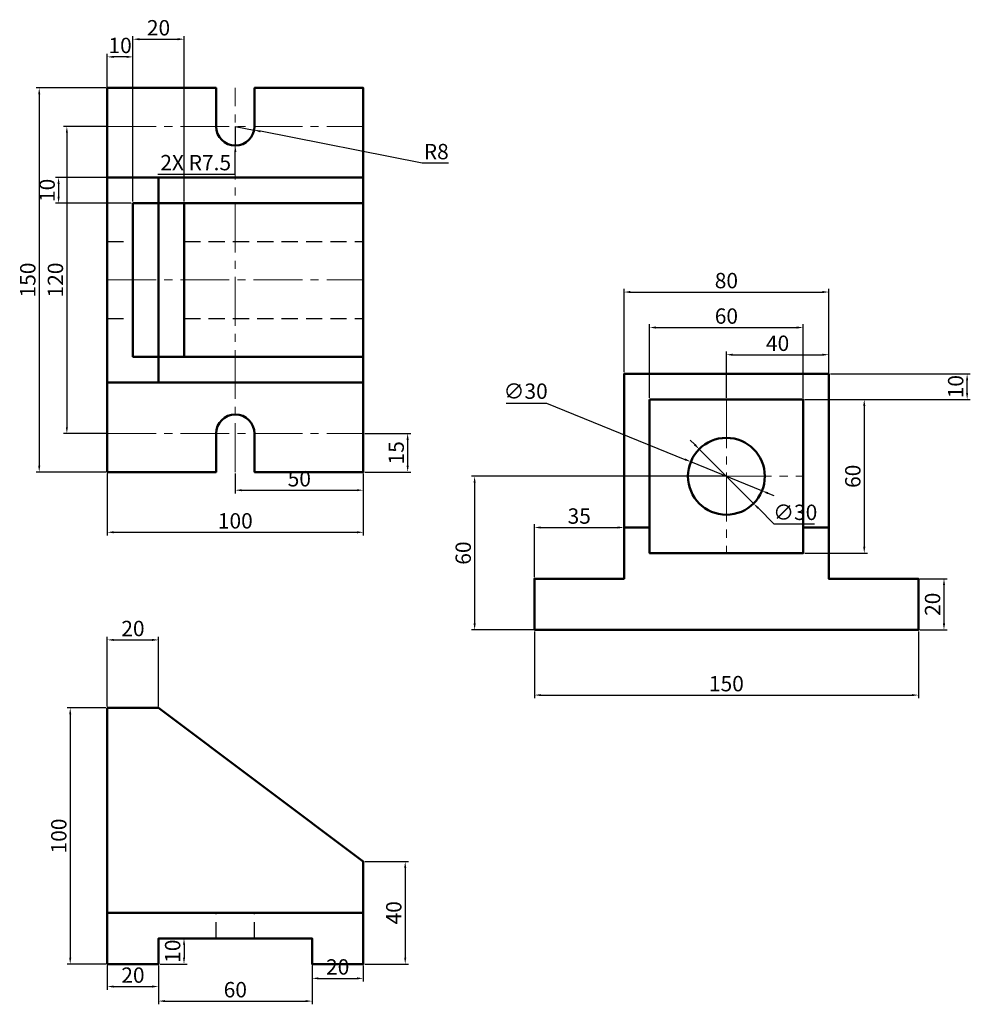
# Model space of a CAD drawing. Units: millimetres. Extents: x 18 to 390, y 656 to 1040.
import ezdxf

# ---------------------------------------------------------------- set-up
doc = ezdxf.new("R2010")
doc.units = ezdxf.units.MM
doc.linetypes.add('CENTER2', pattern=[28.575, 19.05, -3.175, 3.175, -3.175])
doc.linetypes.add('HIDDEN', pattern=[9.525, 6.35, -3.175])
for name, color, linetype, lineweight in [('M-CNTR', 4, 'CENTER2', 18), ('M-DIMS', 2, 'Continuous', 25), ('M-HIDN', 3, 'HIDDEN', 25), ('M-OUTL', 7, 'Continuous', 50)]:
    doc.layers.add(name, color=color, linetype=linetype, lineweight=lineweight)
doc.styles.get("Standard").update_dxf_attribs({"font": 'arial.ttf'})
doc.dimstyles.new('ISO-25', dxfattribs={"dimtxt": 6, "dimasz": 2.5, "dimexe": 1.25, "dimexo": 0.625, "dimtad": 1, "dimtoh": 1, "dimdec": 0, "dimtxsty": 'Standard', "dimcen": 2.5, "dimadec": 0, "dimazin": 0, "dimtfac": 1, "dimtdec": 0, "dimtmove": 0, "dimatfit": 3, "dimfxl": 1, "dimarcsym": 0})

# ---------------------------------------------------------------- blocks, each defined once
blk = doc.blocks.new('*D1')
at = {"layer": 'Defpoints', "color": 0, "transparency": 16777216}
for p in [(102.74, 998.62), (110.1, 997.18)]:
    blk.add_point(p, dxfattribs=at)
at = {"layer": 'M-DIMS', "color": 0, "lineweight": -2, "transparency": 16777216}
for p, q in [((102.74, 998.62), (110.1, 997.18)), ((175.78, 984.31), (112.55, 996.7)), ((186.09, 984.31), (175.78, 984.31))]:
    blk.add_line(p, q, dxfattribs=at)
at = {"layer": 'M-DIMS', "color": 0, "transparency": 16777216}
blk.add_solid([(112.63, 997.11), (112.47, 996.29), (110.1, 997.18)], dxfattribs=at)
at = {"layer": 'M-DIMS', "color": 0, "transparency": 16777216, "insert": (181.25, 988), "char_height": 6, "attachment_point": 5}
blk.add_mtext('R8', dxfattribs=at)
blk = doc.blocks.new('*D2')
at = {"layer": 'Defpoints', "color": 0, "transparency": 16777216}
for p in [(52.74, 1025.77), (52.74, 968.62), (62.74, 968.62)]:
    blk.add_point(p, dxfattribs=at)
at = {"layer": 'M-DIMS', "color": 0, "lineweight": -2, "transparency": 16777216}
for p, q in [((52.74, 969.24), (52.74, 1027.02)), ((62.74, 969.24), (62.74, 1027.02)), ((60.24, 1025.77), (55.24, 1025.77))]:
    blk.add_line(p, q, dxfattribs=at)
at = {"layer": 'M-DIMS', "color": 0, "transparency": 16777216}
for points in [[(55.24, 1026.19), (55.24, 1025.35), (52.74, 1025.77)], [(60.24, 1026.19), (60.24, 1025.35), (62.74, 1025.77)]]:
    blk.add_solid(points, dxfattribs=at)
at = {"layer": 'M-DIMS', "color": 0, "transparency": 16777216, "insert": (57.74, 1029.46), "char_height": 6, "attachment_point": 5}
blk.add_mtext('10', dxfattribs=at)
blk = doc.blocks.new('*D3')
at = {"layer": 'Defpoints', "color": 0, "transparency": 16777216}
for p in [(52.74, 1013.62), (26.13, 863.62), (52.74, 863.62)]:
    blk.add_point(p, dxfattribs=at)
at = {"layer": 'M-DIMS', "color": 0, "lineweight": -2, "transparency": 16777216}
for p, q in [((52.11, 1013.62), (24.88, 1013.62)), ((26.13, 1011.12), (26.13, 866.12)), ((52.11, 863.62), (24.88, 863.62))]:
    blk.add_line(p, q, dxfattribs=at)
at = {"layer": 'M-DIMS', "color": 0, "transparency": 16777216}
for points in [[(25.71, 1011.12), (26.54, 1011.12), (26.13, 1013.62)], [(25.71, 866.12), (26.54, 866.12), (26.13, 863.62)]]:
    blk.add_solid(points, dxfattribs=at)
at = {"layer": 'M-DIMS', "color": 0, "transparency": 16777216, "insert": (22.44, 938.62), "char_height": 6, "attachment_point": 5, "rotation": 90}
blk.add_mtext('150', dxfattribs=at)
blk = doc.blocks.new('*D4')
at = {"layer": 'Defpoints', "color": 0, "transparency": 16777216}
for p in [(52.74, 998.62), (36.93, 878.62), (52.74, 878.62)]:
    blk.add_point(p, dxfattribs=at)
at = {"layer": 'M-DIMS', "color": 0, "lineweight": -2, "transparency": 16777216}
for p, q in [((52.11, 998.62), (35.68, 998.62)), ((36.93, 996.12), (36.93, 881.12)), ((52.11, 878.62), (35.68, 878.62))]:
    blk.add_line(p, q, dxfattribs=at)
at = {"layer": 'M-DIMS', "color": 0, "transparency": 16777216}
for points in [[(36.52, 996.12), (37.35, 996.12), (36.93, 998.62)], [(36.52, 881.12), (37.35, 881.12), (36.93, 878.62)]]:
    blk.add_solid(points, dxfattribs=at)
at = {"layer": 'M-DIMS', "color": 0, "transparency": 16777216, "insert": (33.24, 938.62), "char_height": 6, "attachment_point": 5, "rotation": 90}
blk.add_mtext('120', dxfattribs=at)
blk = doc.blocks.new('*D5')
at = {"layer": 'Defpoints', "color": 0, "transparency": 16777216}
for p in [(102.74, 863.62), (152.74, 863.62), (152.74, 856.52)]:
    blk.add_point(p, dxfattribs=at)
at = {"layer": 'M-DIMS', "color": 0, "lineweight": -2, "transparency": 16777216}
for p, q in [((102.74, 862.99), (102.74, 855.27)), ((152.74, 862.99), (152.74, 855.27)), ((105.24, 856.52), (150.24, 856.52))]:
    blk.add_line(p, q, dxfattribs=at)
at = {"layer": 'M-DIMS', "color": 0, "transparency": 16777216}
for points in [[(105.24, 856.93), (105.24, 856.1), (102.74, 856.52)], [(150.24, 856.93), (150.24, 856.1), (152.74, 856.52)]]:
    blk.add_solid(points, dxfattribs=at)
at = {"layer": 'M-DIMS', "color": 0, "transparency": 16777216, "insert": (127.74, 860.21), "char_height": 6, "attachment_point": 5}
blk.add_mtext('50', dxfattribs=at)
blk = doc.blocks.new('*D6')
at = {"layer": 'Defpoints', "color": 0, "transparency": 16777216}
for p in [(52.74, 863.62), (152.74, 863.62), (152.74, 840.08)]:
    blk.add_point(p, dxfattribs=at)
at = {"layer": 'M-DIMS', "color": 0, "lineweight": -2, "transparency": 16777216}
for p, q in [((52.74, 862.99), (52.74, 838.83)), ((152.74, 862.99), (152.74, 838.83)), ((55.24, 840.08), (150.24, 840.08))]:
    blk.add_line(p, q, dxfattribs=at)
at = {"layer": 'M-DIMS', "color": 0, "transparency": 16777216}
for points in [[(55.24, 840.5), (55.24, 839.66), (52.74, 840.08)], [(150.24, 840.5), (150.24, 839.66), (152.74, 840.08)]]:
    blk.add_solid(points, dxfattribs=at)
at = {"layer": 'M-DIMS', "color": 0, "transparency": 16777216, "insert": (102.74, 843.77), "char_height": 6, "attachment_point": 5}
blk.add_mtext('100', dxfattribs=at)
blk = doc.blocks.new('*D7')
at = {"layer": 'Defpoints', "color": 0, "transparency": 16777216}
for p in [(152.74, 878.62), (152.74, 863.62), (170.07, 863.62)]:
    blk.add_point(p, dxfattribs=at)
at = {"layer": 'M-DIMS', "color": 0, "lineweight": -2, "transparency": 16777216}
for p, q in [((153.36, 878.62), (171.32, 878.62)), ((170.07, 876.12), (170.07, 866.12)), ((153.36, 863.62), (171.32, 863.62))]:
    blk.add_line(p, q, dxfattribs=at)
at = {"layer": 'M-DIMS', "color": 0, "transparency": 16777216}
for points in [[(169.65, 876.12), (170.49, 876.12), (170.07, 878.62)], [(169.65, 866.12), (170.49, 866.12), (170.07, 863.62)]]:
    blk.add_solid(points, dxfattribs=at)
at = {"layer": 'M-DIMS', "color": 0, "transparency": 16777216, "insert": (166.38, 871.12), "char_height": 6, "attachment_point": 5, "rotation": 90}
blk.add_mtext('15', dxfattribs=at)
blk = doc.blocks.new('*D8')
at = {"layer": 'Defpoints', "color": 0, "transparency": 16777216}
for p in [(72.74, 798.04), (52.74, 771.45), (72.74, 771.45)]:
    blk.add_point(p, dxfattribs=at)
at = {"layer": 'M-DIMS', "color": 0, "lineweight": -2, "transparency": 16777216}
for p, q in [((52.74, 772.07), (52.74, 799.29)), ((55.24, 798.04), (70.24, 798.04)), ((72.74, 772.07), (72.74, 799.29))]:
    blk.add_line(p, q, dxfattribs=at)
at = {"layer": 'M-DIMS', "color": 0, "transparency": 16777216}
for points in [[(55.24, 798.45), (55.24, 797.62), (52.74, 798.04)], [(70.24, 798.45), (70.24, 797.62), (72.74, 798.04)]]:
    blk.add_solid(points, dxfattribs=at)
at = {"layer": 'M-DIMS', "color": 0, "transparency": 16777216, "insert": (62.74, 801.72), "char_height": 6, "attachment_point": 5}
blk.add_mtext('20', dxfattribs=at)
blk = doc.blocks.new('*D9')
at = {"layer": 'Defpoints', "color": 0, "transparency": 16777216}
for p in [(52.74, 771.45), (38.25, 671.45), (52.74, 671.45)]:
    blk.add_point(p, dxfattribs=at)
at = {"layer": 'M-DIMS', "color": 0, "lineweight": -2, "transparency": 16777216}
for p, q in [((52.11, 771.45), (37, 771.45)), ((38.25, 768.95), (38.25, 673.95)), ((52.11, 671.45), (37, 671.45))]:
    blk.add_line(p, q, dxfattribs=at)
at = {"layer": 'M-DIMS', "color": 0, "transparency": 16777216}
for points in [[(37.83, 768.95), (38.66, 768.95), (38.25, 771.45)], [(37.83, 673.95), (38.66, 673.95), (38.25, 671.45)]]:
    blk.add_solid(points, dxfattribs=at)
at = {"layer": 'M-DIMS', "color": 0, "transparency": 16777216, "insert": (34.56, 721.45), "char_height": 6, "attachment_point": 5, "rotation": 90}
blk.add_mtext('100', dxfattribs=at)
blk = doc.blocks.new('*D10')
at = {"layer": 'Defpoints', "color": 0, "transparency": 16777216}
for p in [(72.74, 681.45), (72.74, 671.45), (82.7, 671.45)]:
    blk.add_point(p, dxfattribs=at)
at = {"layer": 'M-DIMS', "color": 0, "lineweight": -2, "transparency": 16777216}
for p, q in [((73.36, 681.45), (83.95, 681.45)), ((82.7, 678.95), (82.7, 673.95)), ((73.36, 671.45), (83.95, 671.45))]:
    blk.add_line(p, q, dxfattribs=at)
at = {"layer": 'M-DIMS', "color": 0, "transparency": 16777216}
for points in [[(82.29, 678.95), (83.12, 678.95), (82.7, 681.45)], [(82.29, 673.95), (83.12, 673.95), (82.7, 671.45)]]:
    blk.add_solid(points, dxfattribs=at)
at = {"layer": 'M-DIMS', "color": 0, "transparency": 16777216, "insert": (79.02, 676.45), "char_height": 6, "attachment_point": 5, "rotation": 90}
blk.add_mtext('10', dxfattribs=at)
blk = doc.blocks.new('*D11')
at = {"layer": 'Defpoints', "color": 0, "transparency": 16777216}
for p in [(52.74, 671.45), (72.74, 671.45), (72.74, 662.64)]:
    blk.add_point(p, dxfattribs=at)
at = {"layer": 'M-DIMS', "color": 0, "lineweight": -2, "transparency": 16777216}
for p, q in [((52.74, 670.82), (52.74, 661.39)), ((72.74, 670.82), (72.74, 661.39)), ((55.24, 662.64), (70.24, 662.64))]:
    blk.add_line(p, q, dxfattribs=at)
at = {"layer": 'M-DIMS', "color": 0, "transparency": 16777216}
for points in [[(55.24, 663.06), (55.24, 662.23), (52.74, 662.64)], [(70.24, 663.06), (70.24, 662.23), (72.74, 662.64)]]:
    blk.add_solid(points, dxfattribs=at)
at = {"layer": 'M-DIMS', "color": 0, "transparency": 16777216, "insert": (62.74, 666.33), "char_height": 6, "attachment_point": 5}
blk.add_mtext('20', dxfattribs=at)
blk = doc.blocks.new('*D12')
at = {"layer": 'Defpoints', "color": 0, "transparency": 16777216}
for p in [(72.74, 671.45), (132.74, 671.45), (132.74, 656.96)]:
    blk.add_point(p, dxfattribs=at)
at = {"layer": 'M-DIMS', "color": 0, "lineweight": -2, "transparency": 16777216}
for p, q in [((72.74, 670.82), (72.74, 655.71)), ((132.74, 670.82), (132.74, 655.71)), ((75.24, 656.96), (130.24, 656.96))]:
    blk.add_line(p, q, dxfattribs=at)
at = {"layer": 'M-DIMS', "color": 0, "transparency": 16777216}
for points in [[(75.24, 657.37), (75.24, 656.54), (72.74, 656.96)], [(130.24, 657.37), (130.24, 656.54), (132.74, 656.96)]]:
    blk.add_solid(points, dxfattribs=at)
at = {"layer": 'M-DIMS', "color": 0, "transparency": 16777216, "insert": (102.74, 660.64), "char_height": 6, "attachment_point": 5}
blk.add_mtext('60', dxfattribs=at)
blk = doc.blocks.new('*D13')
at = {"layer": 'Defpoints', "color": 0, "transparency": 16777216}
for p in [(132.74, 671.45), (152.74, 671.45), (152.74, 665.84)]:
    blk.add_point(p, dxfattribs=at)
at = {"layer": 'M-DIMS', "color": 0, "lineweight": -2, "transparency": 16777216}
for p, q in [((132.74, 670.82), (132.74, 664.59)), ((152.74, 670.82), (152.74, 664.59)), ((135.24, 665.84), (150.24, 665.84))]:
    blk.add_line(p, q, dxfattribs=at)
at = {"layer": 'M-DIMS', "color": 0, "transparency": 16777216}
for points in [[(135.24, 666.26), (135.24, 665.42), (132.74, 665.84)], [(150.24, 666.26), (150.24, 665.42), (152.74, 665.84)]]:
    blk.add_solid(points, dxfattribs=at)
at = {"layer": 'M-DIMS', "color": 0, "transparency": 16777216, "insert": (142.74, 669.53), "char_height": 6, "attachment_point": 5}
blk.add_mtext('20', dxfattribs=at)
blk = doc.blocks.new('*D14')
at = {"layer": 'Defpoints', "color": 0, "transparency": 16777216}
for p in [(152.74, 711.45), (152.74, 671.45), (169.13, 671.45)]:
    blk.add_point(p, dxfattribs=at)
at = {"layer": 'M-DIMS', "color": 0, "lineweight": -2, "transparency": 16777216}
for p, q in [((153.36, 711.45), (170.38, 711.45)), ((169.13, 708.95), (169.13, 673.95)), ((153.36, 671.45), (170.38, 671.45))]:
    blk.add_line(p, q, dxfattribs=at)
at = {"layer": 'M-DIMS', "color": 0, "transparency": 16777216}
for points in [[(168.71, 708.95), (169.54, 708.95), (169.13, 711.45)], [(168.71, 673.95), (169.54, 673.95), (169.13, 671.45)]]:
    blk.add_solid(points, dxfattribs=at)
at = {"layer": 'M-DIMS', "color": 0, "transparency": 16777216, "insert": (165.44, 691.45), "char_height": 6, "attachment_point": 5, "rotation": 90}
blk.add_mtext('40', dxfattribs=at)
blk = doc.blocks.new('*D15')
at = {"layer": 'Defpoints', "color": 0, "transparency": 16777216}
for p in [(334.6, 933.92), (254.6, 901.95), (334.6, 901.95)]:
    blk.add_point(p, dxfattribs=at)
at = {"layer": 'M-DIMS', "color": 0, "lineweight": -2, "transparency": 16777216}
for p, q in [((254.6, 902.58), (254.6, 935.17)), ((334.6, 902.58), (334.6, 935.17)), ((257.1, 933.92), (332.1, 933.92))]:
    blk.add_line(p, q, dxfattribs=at)
at = {"layer": 'M-DIMS', "color": 0, "transparency": 16777216}
for points in [[(257.1, 934.34), (257.1, 933.5), (254.6, 933.92)], [(332.1, 934.34), (332.1, 933.5), (334.6, 933.92)]]:
    blk.add_solid(points, dxfattribs=at)
at = {"layer": 'M-DIMS', "color": 0, "transparency": 16777216, "insert": (294.6, 937.61), "char_height": 6, "attachment_point": 5}
blk.add_mtext('80', dxfattribs=at)
blk = doc.blocks.new('*D16')
at = {"layer": 'Defpoints', "color": 0, "transparency": 16777216}
for p in [(324.6, 920.06), (264.6, 891.95), (324.6, 891.95)]:
    blk.add_point(p, dxfattribs=at)
at = {"layer": 'M-DIMS', "color": 0, "lineweight": -2, "transparency": 16777216}
for p, q in [((264.6, 892.58), (264.6, 921.31)), ((267.1, 920.06), (322.1, 920.06)), ((324.6, 892.58), (324.6, 921.31))]:
    blk.add_line(p, q, dxfattribs=at)
at = {"layer": 'M-DIMS', "color": 0, "transparency": 16777216}
for points in [[(267.1, 920.48), (267.1, 919.64), (264.6, 920.06)], [(322.1, 920.48), (322.1, 919.64), (324.6, 920.06)]]:
    blk.add_solid(points, dxfattribs=at)
at = {"layer": 'M-DIMS', "color": 0, "transparency": 16777216, "insert": (294.6, 923.75), "char_height": 6, "attachment_point": 5}
blk.add_mtext('60', dxfattribs=at)
blk = doc.blocks.new('*D17')
at = {"layer": 'Defpoints', "color": 0, "transparency": 16777216}
for p in [(280.7, 867.61), (308.49, 856.29)]:
    blk.add_point(p, dxfattribs=at)
at = {"layer": 'M-DIMS', "color": 0, "lineweight": -2, "transparency": 16777216}
for p, q in [((208.61, 890.57), (224.34, 890.57)), ((224.34, 890.57), (278.39, 868.55)), ((308.49, 856.29), (280.7, 867.61)), ((310.8, 855.35), (313.12, 854.41))]:
    blk.add_line(p, q, dxfattribs=at)
at = {"layer": 'M-DIMS', "color": 0, "transparency": 16777216}
for points in [[(278.55, 868.94), (278.23, 868.17), (280.7, 867.61)], [(310.96, 855.74), (310.65, 854.96), (308.49, 856.29)]]:
    blk.add_solid(points, dxfattribs=at)
at = {"layer": 'M-DIMS', "color": 0, "transparency": 16777216, "insert": (216.16, 894.42), "char_height": 6, "attachment_point": 5}
blk.add_mtext('∅30', dxfattribs=at)
blk = doc.blocks.new('*D18')
at = {"layer": 'Defpoints', "color": 0, "transparency": 16777216}
for p in [(324.6, 891.95), (324.6, 831.95), (348.46, 831.95)]:
    blk.add_point(p, dxfattribs=at)
at = {"layer": 'M-DIMS', "color": 0, "lineweight": -2, "transparency": 16777216}
for p, q in [((325.22, 891.95), (349.71, 891.95)), ((348.46, 889.45), (348.46, 834.45)), ((325.22, 831.95), (349.71, 831.95))]:
    blk.add_line(p, q, dxfattribs=at)
at = {"layer": 'M-DIMS', "color": 0, "transparency": 16777216}
for points in [[(348.04, 889.45), (348.88, 889.45), (348.46, 891.95)], [(348.04, 834.45), (348.88, 834.45), (348.46, 831.95)]]:
    blk.add_solid(points, dxfattribs=at)
at = {"layer": 'M-DIMS', "color": 0, "transparency": 16777216, "insert": (344.77, 861.95), "char_height": 6, "attachment_point": 5, "rotation": 90}
blk.add_mtext('60', dxfattribs=at)
blk = doc.blocks.new('*D19')
at = {"layer": 'Defpoints', "color": 0, "transparency": 16777216}
for p in [(254.6, 841.95), (219.6, 821.95), (254.6, 821.95)]:
    blk.add_point(p, dxfattribs=at)
at = {"layer": 'M-DIMS', "color": 0, "lineweight": -2, "transparency": 16777216}
for p, q in [((219.6, 822.58), (219.6, 843.2)), ((254.6, 822.58), (254.6, 843.2)), ((222.1, 841.95), (252.1, 841.95))]:
    blk.add_line(p, q, dxfattribs=at)
at = {"layer": 'M-DIMS', "color": 0, "transparency": 16777216}
for points in [[(222.1, 842.37), (222.1, 841.53), (219.6, 841.95)], [(252.1, 842.37), (252.1, 841.53), (254.6, 841.95)]]:
    blk.add_solid(points, dxfattribs=at)
at = {"layer": 'M-DIMS', "color": 0, "transparency": 16777216, "insert": (237.1, 845.64), "char_height": 6, "attachment_point": 5}
blk.add_mtext('35', dxfattribs=at)
blk = doc.blocks.new('*D20')
at = {"layer": 'Defpoints', "color": 0, "transparency": 16777216}
for p in [(294.6, 861.95), (196.24, 801.95), (294.6, 801.95)]:
    blk.add_point(p, dxfattribs=at)
at = {"layer": 'M-DIMS', "color": 0, "lineweight": -2, "transparency": 16777216}
for p, q in [((293.97, 861.95), (194.99, 861.95)), ((196.24, 859.45), (196.24, 804.45)), ((293.97, 801.95), (194.99, 801.95))]:
    blk.add_line(p, q, dxfattribs=at)
at = {"layer": 'M-DIMS', "color": 0, "transparency": 16777216}
for points in [[(195.82, 859.45), (196.65, 859.45), (196.24, 861.95)], [(195.82, 804.45), (196.65, 804.45), (196.24, 801.95)]]:
    blk.add_solid(points, dxfattribs=at)
at = {"layer": 'M-DIMS', "color": 0, "transparency": 16777216, "insert": (192.55, 831.95), "char_height": 6, "attachment_point": 5, "rotation": 90}
blk.add_mtext('60', dxfattribs=at)
blk = doc.blocks.new('*D21')
at = {"layer": 'Defpoints', "color": 0, "transparency": 16777216}
for p in [(369.6, 821.95), (369.6, 801.95), (379.61, 801.95)]:
    blk.add_point(p, dxfattribs=at)
at = {"layer": 'M-DIMS', "color": 0, "lineweight": -2, "transparency": 16777216}
for p, q in [((370.22, 821.95), (380.86, 821.95)), ((379.61, 819.45), (379.61, 804.45)), ((370.22, 801.95), (380.86, 801.95))]:
    blk.add_line(p, q, dxfattribs=at)
at = {"layer": 'M-DIMS', "color": 0, "transparency": 16777216}
for points in [[(379.19, 819.45), (380.03, 819.45), (379.61, 821.95)], [(379.19, 804.45), (380.03, 804.45), (379.61, 801.95)]]:
    blk.add_solid(points, dxfattribs=at)
at = {"layer": 'M-DIMS', "color": 0, "transparency": 16777216, "insert": (375.92, 811.95), "char_height": 6, "attachment_point": 5, "rotation": 90}
blk.add_mtext('20', dxfattribs=at)
blk = doc.blocks.new('*D22')
at = {"layer": 'Defpoints', "color": 0, "transparency": 16777216}
for p in [(219.6, 801.95), (369.6, 801.95), (369.6, 776.49)]:
    blk.add_point(p, dxfattribs=at)
at = {"layer": 'M-DIMS', "color": 0, "lineweight": -2, "transparency": 16777216}
for p, q in [((219.6, 801.33), (219.6, 775.24)), ((369.6, 801.33), (369.6, 775.24)), ((222.1, 776.49), (367.1, 776.49))]:
    blk.add_line(p, q, dxfattribs=at)
at = {"layer": 'M-DIMS', "color": 0, "transparency": 16777216}
for points in [[(222.1, 776.9), (222.1, 776.07), (219.6, 776.49)], [(367.1, 776.9), (367.1, 776.07), (369.6, 776.49)]]:
    blk.add_solid(points, dxfattribs=at)
at = {"layer": 'M-DIMS', "color": 0, "transparency": 16777216, "insert": (294.6, 780.18), "char_height": 6, "attachment_point": 5}
blk.add_mtext('150', dxfattribs=at)
blk = doc.blocks.new('*D23')
at = {"layer": 'Defpoints', "color": 0, "transparency": 16777216}
for p in [(334.6, 909.44), (334.6, 894.75), (294.6, 891.95)]:
    blk.add_point(p, dxfattribs=at)
at = {"layer": 'M-DIMS', "color": 0, "lineweight": -2, "transparency": 16777216}
for p, q in [((294.6, 892.58), (294.6, 910.69)), ((297.1, 909.44), (332.1, 909.44)), ((334.6, 895.37), (334.6, 910.69))]:
    blk.add_line(p, q, dxfattribs=at)
at = {"layer": 'M-DIMS', "color": 0, "transparency": 16777216}
for points in [[(297.1, 909.85), (297.1, 909.02), (294.6, 909.44)], [(332.1, 909.85), (332.1, 909.02), (334.6, 909.44)]]:
    blk.add_solid(points, dxfattribs=at)
at = {"layer": 'M-DIMS', "color": 0, "transparency": 16777216, "insert": (314.6, 913.13), "char_height": 6, "attachment_point": 5}
blk.add_mtext('40', dxfattribs=at)
blk = doc.blocks.new('*D24')
at = {"layer": 'Defpoints', "color": 0, "transparency": 16777216}
for p in [(334.6, 901.95), (388.65, 901.95), (324.6, 891.95)]:
    blk.add_point(p, dxfattribs=at)
at = {"layer": 'M-DIMS', "color": 0, "lineweight": -2, "transparency": 16777216}
for p, q in [((335.22, 901.95), (389.9, 901.95)), ((388.65, 894.45), (388.65, 899.45)), ((325.22, 891.95), (389.9, 891.95))]:
    blk.add_line(p, q, dxfattribs=at)
at = {"layer": 'M-DIMS', "color": 0, "transparency": 16777216}
for points in [[(388.23, 899.45), (389.06, 899.45), (388.65, 901.95)], [(388.23, 894.45), (389.06, 894.45), (388.65, 891.95)]]:
    blk.add_solid(points, dxfattribs=at)
at = {"layer": 'M-DIMS', "color": 0, "transparency": 16777216, "insert": (384.96, 896.95), "char_height": 6, "attachment_point": 5, "rotation": 90}
blk.add_mtext('10', dxfattribs=at)
blk = doc.blocks.new('*D25')
at = {"layer": 'Defpoints', "color": 0, "transparency": 16777216}
for p in [(52.74, 978.62), (33.69, 968.62), (62.74, 968.62)]:
    blk.add_point(p, dxfattribs=at)
at = {"layer": 'M-DIMS', "color": 0, "lineweight": -2, "transparency": 16777216}
for p, q in [((52.11, 978.62), (32.44, 978.62)), ((33.69, 976.12), (33.69, 971.12)), ((62.11, 968.62), (32.44, 968.62))]:
    blk.add_line(p, q, dxfattribs=at)
at = {"layer": 'M-DIMS', "color": 0, "transparency": 16777216}
for points in [[(33.27, 976.12), (34.11, 976.12), (33.69, 978.62)], [(33.27, 971.12), (34.11, 971.12), (33.69, 968.62)]]:
    blk.add_solid(points, dxfattribs=at)
at = {"layer": 'M-DIMS', "color": 0, "transparency": 16777216, "insert": (30, 973.62), "char_height": 6, "attachment_point": 5, "rotation": 90}
blk.add_mtext('10', dxfattribs=at)
blk = doc.blocks.new('*D26')
at = {"layer": 'Defpoints', "color": 0, "transparency": 16777216}
for p in [(82.74, 1032.67), (62.74, 968.62), (82.74, 968.62)]:
    blk.add_point(p, dxfattribs=at)
at = {"layer": 'M-DIMS', "color": 0, "lineweight": -2, "transparency": 16777216}
for p, q in [((62.74, 969.24), (62.74, 1033.92)), ((65.24, 1032.67), (80.24, 1032.67)), ((82.74, 969.24), (82.74, 1033.92))]:
    blk.add_line(p, q, dxfattribs=at)
at = {"layer": 'M-DIMS', "color": 0, "transparency": 16777216}
for points in [[(65.24, 1033.09), (65.24, 1032.25), (62.74, 1032.67)], [(80.24, 1033.09), (80.24, 1032.25), (82.74, 1032.67)]]:
    blk.add_solid(points, dxfattribs=at)
at = {"layer": 'M-DIMS', "color": 0, "transparency": 16777216, "insert": (72.74, 1036.36), "char_height": 6, "attachment_point": 5}
blk.add_mtext('20', dxfattribs=at)
blk = doc.blocks.new('*D27')
at = {"layer": 'Defpoints', "color": 0, "transparency": 16777216}
for p in [(283.99, 872.56), (305.2, 851.34)]:
    blk.add_point(p, dxfattribs=at)
at = {"layer": 'M-DIMS', "color": 0, "lineweight": -2, "transparency": 16777216}
for p, q in [((282.22, 874.33), (280.45, 876.09)), ((283.99, 872.56), (305.2, 851.34)), ((313.31, 843.24), (306.97, 849.58)), ((329.03, 843.24), (313.31, 843.24))]:
    blk.add_line(p, q, dxfattribs=at)
at = {"layer": 'M-DIMS', "color": 0, "transparency": 16777216}
for points in [[(282.52, 874.62), (281.93, 874.03), (283.99, 872.56)], [(307.26, 849.87), (306.68, 849.28), (305.2, 851.34)]]:
    blk.add_solid(points, dxfattribs=at)
at = {"layer": 'M-DIMS', "color": 0, "transparency": 16777216, "insert": (321.48, 847.1), "char_height": 6, "attachment_point": 5}
blk.add_mtext('∅30', dxfattribs=at)
blk = doc.blocks.new('*D28')
at = {"layer": 'Defpoints', "color": 0, "transparency": 16777216}
for p in [(102.74, 998.62), (102.74, 991.12)]:
    blk.add_point(p, dxfattribs=at)
at = {"layer": 'M-DIMS', "color": 0, "lineweight": -2, "transparency": 16777216}
for p, q in [((102.74, 998.62), (102.74, 991.12)), ((102.74, 979.99), (102.74, 988.62)), ((72.41, 979.99), (102.74, 979.99))]:
    blk.add_line(p, q, dxfattribs=at)
at = {"layer": 'M-DIMS', "color": 0, "transparency": 16777216}
blk.add_solid([(102.32, 988.62), (103.16, 988.62), (102.74, 991.12)], dxfattribs=at)
at = {"layer": 'M-DIMS', "color": 0, "transparency": 16777216, "insert": (87.26, 983.68), "char_height": 6, "attachment_point": 5}
blk.add_mtext('2X R7.5', dxfattribs=at)

msp = doc.modelspace()

# ---------------------------------------------------------------- linework, layer by layer
at = {"layer": 'M-CNTR'}
for p, q in [((102.74, 863.62), (102.74, 1013.62)), ((52.74, 998.62), (152.74, 998.62)), ((52.74, 938.62), (152.74, 938.62)), ((294.6, 891.95), (294.6, 831.95)), ((52.74, 878.62), (152.74, 878.62)), ((264.6, 861.95), (324.6, 861.95))]:
    msp.add_line(p, q, dxfattribs=at)
at = {"layer": 'M-HIDN'}
for p, q in [((52.74, 953.62), (62.74, 953.62)), ((82.74, 953.62), (152.74, 953.62)), ((52.74, 923.62), (62.74, 923.62)), ((82.74, 923.62), (152.74, 923.62)), ((95.24, 681.45), (95.24, 691.45)), ((110.24, 681.45), (110.24, 691.45))]:
    msp.add_line(p, q, dxfattribs=at)
at = {"layer": 'M-OUTL'}
for p, q in [((52.74, 978.62), (152.74, 978.62)), ((72.74, 978.62), (72.74, 898.62)), ((82.74, 968.62), (82.74, 908.62)), ((52.74, 898.62), (152.74, 898.62)), ((254.6, 841.95), (264.6, 841.95)), ((334.6, 841.95), (324.6, 841.95)), ((52.74, 691.45), (152.74, 691.45))]:
    msp.add_line(p, q, dxfattribs=at)
msp.add_lwpolyline([(52.74, 1013.62), (52.74, 863.62), (95.24, 863.62), (95.24, 878.62, -1), (110.24, 878.62), (110.24, 863.62), (152.74, 863.62), (152.74, 1013.62), (110.24, 1013.62), (110.24, 998.62, -1), (95.24, 998.62), (95.24, 1013.62)], format="xyb", close=True, dxfattribs=at)
msp.add_lwpolyline([(152.74, 908.62), (62.74, 908.62), (62.74, 968.62), (152.74, 968.62)], dxfattribs=at)
for points in [[(219.6, 801.95), (219.6, 821.95), (254.6, 821.95), (254.6, 901.95), (334.6, 901.95), (334.6, 821.95), (369.6, 821.95), (369.6, 801.95)], [(264.6, 891.95), (324.6, 891.95), (324.6, 831.95), (264.6, 831.95)], [(52.74, 771.45), (72.74, 771.45), (152.74, 711.45), (152.74, 671.45), (132.74, 671.45), (132.74, 681.45), (72.74, 681.45), (72.74, 671.45), (52.74, 671.45)]]:
    msp.add_lwpolyline(points, close=True, dxfattribs=at)
msp.add_circle((294.6, 861.95), 15, dxfattribs=at)

# ---------------------------------------------------------------- dimensions: what is measured, and where the dimension line sits
at = {"layer": 'M-DIMS'}
for base, p1, p2, override, picture, middle in [((82.74, 1032.67), (62.74, 968.62), (82.74, 968.62), {"dimdec": 0, "dimlfac": 1, "dimrnd": 0, "dimzin": 0, "dimdsep": 46, "dimlunit": 2}, '*D26', (72.74, 1036.36)), ((52.74, 1025.77), (62.74, 968.62), (52.74, 968.62), {"dimclrd": 0, "dimclre": 0, "dimclrt": 0}, '*D2', (57.74, 1029.46)), ((334.6, 933.92), (254.6, 901.95), (334.6, 901.95), {"dimclrd": 0, "dimclre": 0, "dimclrt": 0}, '*D15', (294.6, 937.61)), ((324.6, 920.06), (264.6, 891.95), (324.6, 891.95), {"dimclrd": 0, "dimclre": 0, "dimclrt": 0}, '*D16', (294.6, 923.75)), ((334.6, 909.44), (294.6, 891.95), (334.6, 894.75), {"dimclrd": 0, "dimclre": 0, "dimclrt": 0}, '*D23', (314.6, 913.13)), ((152.74, 840.08), (52.74, 863.62), (152.74, 863.62), {"dimclrd": 0, "dimclre": 0, "dimclrt": 0}, '*D6', (102.74, 843.77)), ((152.74, 856.52), (102.74, 863.62), (152.74, 863.62), {"dimclrd": 0, "dimclre": 0, "dimclrt": 0}, '*D5', (127.74, 860.21)), ((254.6, 841.95), (219.6, 821.95), (254.6, 821.95), {"dimclrd": 0, "dimclre": 0, "dimclrt": 0}, '*D19', (237.1, 845.64)), ((72.74, 798.04), (52.74, 771.45), (72.74, 771.45), {"dimclrd": 0, "dimclre": 0, "dimclrt": 0}, '*D8', (62.74, 801.72)), ((369.6, 776.49), (219.6, 801.95), (369.6, 801.95), {"dimclrd": 0, "dimclre": 0, "dimclrt": 0}, '*D22', (294.6, 780.18)), ((152.74, 665.84), (132.74, 671.45), (152.74, 671.45), {"dimclrd": 0, "dimclre": 0, "dimclrt": 0}, '*D13', (142.74, 669.53)), ((72.74, 662.64), (52.74, 671.45), (72.74, 671.45), {"dimclrd": 0, "dimclre": 0, "dimclrt": 0}, '*D11', (62.74, 666.33)), ((132.74, 656.96), (72.74, 671.45), (132.74, 671.45), {"dimclrd": 0, "dimclre": 0, "dimclrt": 0}, '*D12', (102.74, 660.64))]:
    dim = msp.add_linear_dim(base=base, p1=p1, p2=p2, dimstyle='ISO-25', override=override, dxfattribs=at)
    dim.commit()
    dim.dimension.update_dxf_attribs({"geometry": picture, "text_midpoint": middle})
for base, p1, p2, override, picture, middle in [((26.13, 863.62), (52.74, 1013.62), (52.74, 863.62), {"dimclrd": 0, "dimclre": 0, "dimclrt": 0}, '*D3', (22.44, 938.62)), ((36.93, 878.62), (52.74, 998.62), (52.74, 878.62), {"dimclrd": 0, "dimclre": 0, "dimclrt": 0}, '*D4', (33.24, 938.62)), ((33.69, 968.62), (52.74, 978.62), (62.74, 968.62), {"dimdec": 0, "dimlfac": 1, "dimrnd": 0, "dimzin": 0, "dimdsep": 46, "dimlunit": 2}, '*D25', (30, 973.62)), ((388.65, 901.95), (324.6, 891.95), (334.6, 901.95), {"dimdec": 0, "dimlfac": 1, "dimrnd": 0, "dimzin": 0, "dimdsep": 46, "dimlunit": 2}, '*D24', (384.96, 896.95)), ((348.46, 831.95), (324.6, 891.95), (324.6, 831.95), {"dimclrd": 0, "dimclre": 0, "dimclrt": 0}, '*D18', (344.77, 861.95)), ((170.07, 863.62), (152.74, 878.62), (152.74, 863.62), {"dimclrd": 0, "dimclre": 0, "dimclrt": 0}, '*D7', (166.38, 871.12)), ((196.24, 801.95), (294.6, 861.95), (294.6, 801.95), {"dimclrd": 0, "dimclre": 0, "dimclrt": 0}, '*D20', (192.55, 831.95)), ((379.61, 801.95), (369.6, 821.95), (369.6, 801.95), {"dimclrd": 0, "dimclre": 0, "dimclrt": 0}, '*D21', (375.92, 811.95)), ((38.25, 671.45), (52.74, 771.45), (52.74, 671.45), {"dimclrd": 0, "dimclre": 0, "dimclrt": 0}, '*D9', (34.56, 721.45)), ((169.13, 671.45), (152.74, 711.45), (152.74, 671.45), {"dimclrd": 0, "dimclre": 0, "dimclrt": 0}, '*D14', (165.44, 691.45)), ((82.7, 671.45), (72.74, 681.45), (72.74, 671.45), {"dimclrd": 0, "dimclre": 0, "dimclrt": 0}, '*D10', (79.02, 676.45))]:
    dim = msp.add_linear_dim(base=base, p1=p1, p2=p2, angle=90, dimstyle='ISO-25', override=override, dxfattribs=at)
    dim.commit()
    dim.dimension.update_dxf_attribs({"geometry": picture, "text_midpoint": middle})
dim = msp.add_radius_dim(center=(102.74, 998.62), mpoint=(102.74, 991.12), text='2X <>', dimstyle='ISO-25', override={"dimdec": 1, "dimlfac": 1, "dimrnd": 0, "dimzin": 0, "dimdsep": 46, "dimlunit": 2}, dxfattribs=at)
dim.commit()
dim.dimension.update_dxf_attribs({"geometry": '*D28', "text_midpoint": (87.26, 983.68)})
dim = msp.add_radius_dim(center=(102.739, 998.6191), mpoint=(110.0992, 997.1776), dimstyle='ISO-25', override={"dimclrd": 0, "dimclre": 0, "dimclrt": 0}, dxfattribs=at)
dim.commit()
dim.dimension.update_dxf_attribs({"geometry": '*D1', "text_midpoint": (175.782, 984.3135), "dimtype": 164})
dim = msp.add_diameter_dim_2p(p1=(308.49, 856.29), p2=(280.7, 867.61), dimstyle='ISO-25', override={"dimclrd": 0, "dimclre": 0, "dimclrt": 0}, dxfattribs=at)
dim.commit()
dim.dimension.update_dxf_attribs({"geometry": '*D17', "text_midpoint": (216.16, 890.57), "dimtype": 163})
dim = msp.add_diameter_dim_2p(p1=(283.99, 872.56), p2=(305.2, 851.34), dimstyle='ISO-25', override={"dimdec": 0, "dimlfac": 1, "dimrnd": 0, "dimzin": 0, "dimdsep": 46, "dimlunit": 2}, dxfattribs=at)
dim.commit()
dim.dimension.update_dxf_attribs({"geometry": '*D27', "text_midpoint": (321.48, 843.24)})

doc.saveas('drawing.dxf')
